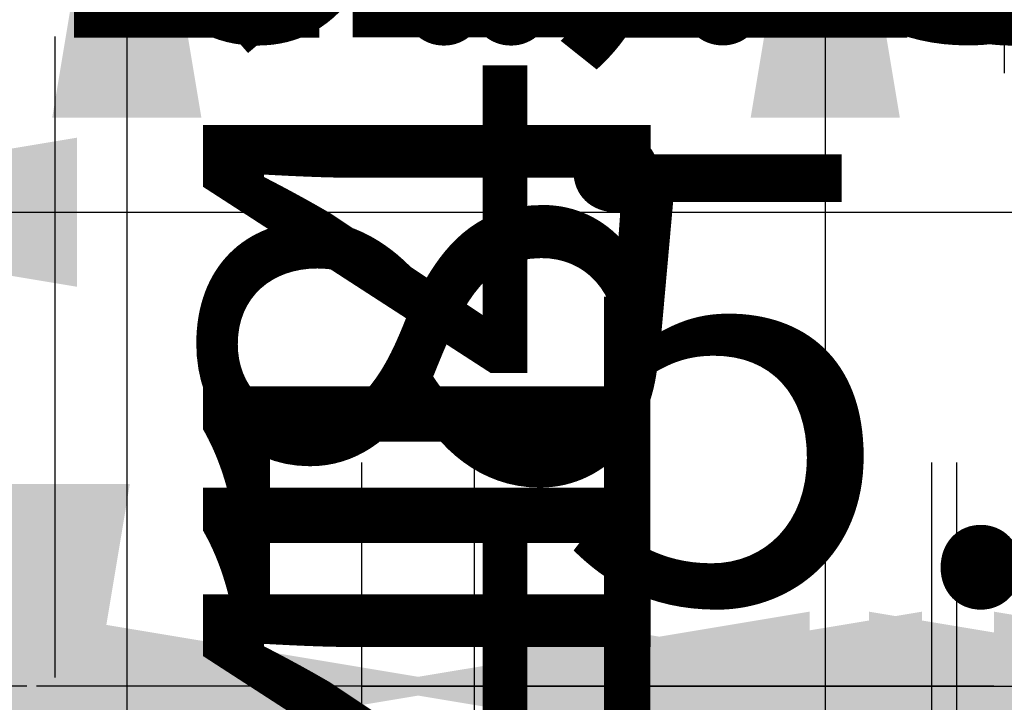
# Model space of a CAD drawing. Units: metres. Extents: x 782 to 1487, y 1262 to 7446.
# Tile 11 of 25: x 834.592 to 840.091, y 1284.539 to 1288.353. Entities that reach past the tile are written whole.
import ezdxf

# ---------------------------------------------------------------- set-up
doc = ezdxf.new("R2010")
doc.units = ezdxf.units.M
doc.layers.add('A-ANNO-DIMS', color=2, linetype='Continuous', lineweight=18)
doc.styles.get("Standard").update_dxf_attribs({"font": 'arial.ttf'})
doc.dimstyles.new('ISO-25', dxfattribs={"dimtxt": 2.5, "dimasz": 2.5, "dimexe": 1.25, "dimexo": 0.625, "dimtad": 1, "dimtxsty": 'Standard', "dimcen": 2.5, "dimadec": 0, "dimazin": 0, "dimtfac": 1, "dimtmove": 0, "dimatfit": 3, "dimfxl": 1, "dimarcsym": 0})

# ---------------------------------------------------------------- blocks, each defined once
blk = doc.blocks.new('*D88')
at = {"layer": 'A-ANNO-DIMS', "color": 0, "lineweight": -2, "transparency": 16777216}
for p, q in [((835.1905, 1307.3669), (835.1905, 1309.8669)), ((833.0382, 1304.8669), (836.4405, 1304.8669)), ((835.1905, 1304.8669), (835.1905, 1300.3378)), ((833.0381, 1300.3378), (836.4405, 1300.3378)), ((835.1905, 1297.8378), (835.1905, 1285.5459))]:
    blk.add_line(p, q, dxfattribs=at)
at = {"layer": 'A-ANNO-DIMS', "color": 0, "transparency": 16777216}
for points in [[(834.7738, 1307.3669), (835.6071, 1307.3669), (835.1905, 1304.8669)], [(834.7738, 1297.8378), (835.6071, 1297.8378), (835.1905, 1300.3378)]]:
    blk.add_solid(points, dxfattribs=at)
at = {"layer": 'Defpoints', "color": 0, "transparency": 16777216}
for p in [(832.4132, 1304.8669), (832.4131, 1300.3378), (835.1905, 1300.3378)]:
    blk.add_point(p, dxfattribs=at)
at = {"layer": 'A-ANNO-DIMS', "color": 0, "transparency": 16777216, "insert": (833.289, 1290.4419), "char_height": 2.5, "attachment_point": 5, "rotation": 90}
blk.add_mtext('4.529', dxfattribs=at)
blk = doc.blocks.new('*D89')
at = {"layer": 'A-ANNO-DIMS', "color": 0, "lineweight": -2, "transparency": 16777216}
for p, q in [((835.1905, 1302.8378), (835.1905, 1305.3378)), ((833.0381, 1300.3378), (836.4405, 1300.3378)), ((835.1905, 1300.3378), (835.1905, 1296.196)), ((833.0375, 1296.196), (836.4405, 1296.196)), ((835.1905, 1293.696), (835.1905, 1281.4347))]:
    blk.add_line(p, q, dxfattribs=at)
at = {"layer": 'A-ANNO-DIMS', "color": 0, "transparency": 16777216}
for points in [[(834.7738, 1302.8378), (835.6071, 1302.8378), (835.1905, 1300.3378)], [(834.7738, 1293.696), (835.6071, 1293.696), (835.1905, 1296.196)]]:
    blk.add_solid(points, dxfattribs=at)
at = {"layer": 'Defpoints', "color": 0, "transparency": 16777216}
for p in [(832.4131, 1300.3378), (832.4125, 1296.196), (835.1905, 1296.196)]:
    blk.add_point(p, dxfattribs=at)
at = {"layer": 'A-ANNO-DIMS', "color": 0, "transparency": 16777216, "insert": (833.3103, 1286.3153), "char_height": 2.5, "attachment_point": 5, "rotation": 90}
blk.add_mtext('4.142', dxfattribs=at)
blk = doc.blocks.new('*D90')
at = {"layer": 'A-ANNO-DIMS', "color": 0, "lineweight": -2, "transparency": 16777216}
for p, q in [((835.1905, 1298.696), (835.1905, 1301.196)), ((833.0375, 1296.196), (836.4405, 1296.196)), ((835.1905, 1296.196), (835.1905, 1293.6994)), ((833.0375, 1293.6994), (836.4405, 1293.6994)), ((835.1905, 1291.1994), (835.1905, 1280.9214))]:
    blk.add_line(p, q, dxfattribs=at)
at = {"layer": 'A-ANNO-DIMS', "color": 0, "transparency": 16777216}
for points in [[(834.7738, 1298.696), (835.6071, 1298.696), (835.1905, 1296.196)], [(834.7738, 1291.1994), (835.6071, 1291.1994), (835.1905, 1293.6994)]]:
    blk.add_solid(points, dxfattribs=at)
at = {"layer": 'Defpoints', "color": 0, "transparency": 16777216}
for p in [(832.4125, 1296.196), (832.4125, 1293.6994), (835.1905, 1293.6994)]:
    blk.add_point(p, dxfattribs=at)
at = {"layer": 'A-ANNO-DIMS', "color": 0, "transparency": 16777216, "insert": (833.289, 1284.8104), "char_height": 2.5, "attachment_point": 5, "rotation": 90}
blk.add_mtext('2.50', dxfattribs=at)
blk = doc.blocks.new('*D91')
at = {"layer": 'A-ANNO-DIMS', "color": 0, "lineweight": -2, "transparency": 16777216}
for p, q in [((835.1905, 1296.1994), (835.1905, 1298.6994)), ((833.0375, 1293.6994), (836.4405, 1293.6994)), ((835.1905, 1293.6994), (835.1905, 1293.0674)), ((833.0375, 1293.0674), (836.4405, 1293.0674)), ((835.1905, 1290.5674), (835.1905, 1278.4068))]:
    blk.add_line(p, q, dxfattribs=at)
at = {"layer": 'A-ANNO-DIMS', "color": 0, "transparency": 16777216}
for points in [[(834.7738, 1296.1994), (835.6071, 1296.1994), (835.1905, 1293.6994)], [(834.7738, 1290.5674), (835.6071, 1290.5674), (835.1905, 1293.0674)]]:
    blk.add_solid(points, dxfattribs=at)
at = {"layer": 'Defpoints', "color": 0, "transparency": 16777216}
for p in [(832.4125, 1293.6994), (832.4125, 1293.0674), (835.1905, 1293.0674)]:
    blk.add_point(p, dxfattribs=at)
at = {"layer": 'A-ANNO-DIMS', "color": 0, "transparency": 16777216, "insert": (833.2882, 1283.2371), "char_height": 2.5, "attachment_point": 5, "rotation": 90}
blk.add_mtext('0.632', dxfattribs=at)
blk = doc.blocks.new('*D92')
at = {"layer": 'A-ANNO-DIMS', "color": 0, "lineweight": -2, "transparency": 16777216}
for p, q in [((835.1905, 1295.5674), (835.1905, 1298.0674)), ((831.3406, 1293.0674), (836.4405, 1293.0674)), ((835.1905, 1293.0674), (835.1905, 1291.6863)), ((831.3406, 1291.6863), (836.4405, 1291.6863)), ((835.1905, 1289.1863), (835.1905, 1277.7181))]:
    blk.add_line(p, q, dxfattribs=at)
at = {"layer": 'A-ANNO-DIMS', "color": 0, "transparency": 16777216}
for points in [[(834.7738, 1295.5674), (835.6071, 1295.5674), (835.1905, 1293.0674)], [(834.7738, 1289.1863), (835.6071, 1289.1863), (835.1905, 1291.6863)]]:
    blk.add_solid(points, dxfattribs=at)
at = {"layer": 'Defpoints', "color": 0, "transparency": 16777216}
for p in [(830.7156, 1293.0674), (830.7156, 1291.6863), (835.1905, 1291.6863)]:
    blk.add_point(p, dxfattribs=at)
at = {"layer": 'A-ANNO-DIMS', "color": 0, "transparency": 16777216, "insert": (833.2882, 1282.2022), "char_height": 2.5, "attachment_point": 5, "rotation": 90}
blk.add_mtext('1.381', dxfattribs=at)
blk = doc.blocks.new('*D93')
at = {"layer": 'A-ANNO-DIMS', "color": 0, "lineweight": -2, "transparency": 16777216}
for p, q in [((835.1905, 1294.1863), (835.1905, 1296.6863)), ((831.3406, 1291.6863), (836.4405, 1291.6863)), ((835.1905, 1291.6863), (835.1905, 1290.3053)), ((831.3406, 1290.3053), (836.4405, 1290.3053)), ((835.1905, 1287.8053), (835.1905, 1276.337))]:
    blk.add_line(p, q, dxfattribs=at)
at = {"layer": 'A-ANNO-DIMS', "color": 0, "transparency": 16777216}
for points in [[(834.7738, 1294.1863), (835.6071, 1294.1863), (835.1905, 1291.6863)], [(834.7738, 1287.8053), (835.6071, 1287.8053), (835.1905, 1290.3053)]]:
    blk.add_solid(points, dxfattribs=at)
at = {"layer": 'Defpoints', "color": 0, "transparency": 16777216}
for p in [(830.7156, 1291.6863), (830.7156, 1290.3053), (835.1905, 1290.3053)]:
    blk.add_point(p, dxfattribs=at)
at = {"layer": 'A-ANNO-DIMS', "color": 0, "transparency": 16777216, "insert": (833.2882, 1280.8211), "char_height": 2.5, "attachment_point": 5, "rotation": 90}
blk.add_mtext('1.381', dxfattribs=at)
blk = doc.blocks.new('*D97')
at = {"layer": 'A-ANNO-DIMS', "color": 0, "lineweight": -2, "transparency": 16777216}
for p, q in [((827.9625, 1289.6803), (827.9625, 1286.0275)), ((829.1513, 1289.6803), (829.1513, 1286.0275)), ((825.4625, 1287.2775), (822.9625, 1287.2775)), ((827.9625, 1287.2775), (829.1513, 1287.2775)), ((831.6513, 1287.2775), (841.6649, 1287.2775))]:
    blk.add_line(p, q, dxfattribs=at)
at = {"layer": 'A-ANNO-DIMS', "color": 0, "transparency": 16777216}
for points in [[(825.4625, 1287.6941), (825.4625, 1286.8608), (827.9625, 1287.2775)], [(831.6513, 1287.6941), (831.6513, 1286.8608), (829.1513, 1287.2775)]]:
    blk.add_solid(points, dxfattribs=at)
at = {"layer": 'Defpoints', "color": 0, "transparency": 16777216}
for p in [(827.9625, 1290.3053), (829.1513, 1290.3053), (829.1513, 1287.2775)]:
    blk.add_point(p, dxfattribs=at)
at = {"layer": 'A-ANNO-DIMS', "color": 0, "transparency": 16777216, "insert": (837.9081, 1289.1789), "char_height": 2.5, "attachment_point": 5}
blk.add_mtext('1.19', dxfattribs=at)
blk = doc.blocks.new('*D98')
at = {"layer": 'A-ANNO-DIMS', "color": 0, "lineweight": -2, "transparency": 16777216}
for p, q in [((829.1513, 1289.6803), (829.1513, 1286.0275)), ((829.412, 1289.6803), (829.412, 1286.0275)), ((826.6513, 1287.2775), (824.1513, 1287.2775)), ((829.1513, 1287.2775), (829.412, 1287.2775)), ((831.912, 1287.2775), (842.1542, 1287.2775))]:
    blk.add_line(p, q, dxfattribs=at)
at = {"layer": 'A-ANNO-DIMS', "color": 0, "transparency": 16777216}
for points in [[(826.6513, 1287.6941), (826.6513, 1286.8608), (829.1513, 1287.2775)], [(831.912, 1287.6941), (831.912, 1286.8608), (829.412, 1287.2775)]]:
    blk.add_solid(points, dxfattribs=at)
at = {"layer": 'Defpoints', "color": 0, "transparency": 16777216}
for p in [(829.1513, 1290.3053), (829.412, 1290.3053), (829.412, 1287.2775)]:
    blk.add_point(p, dxfattribs=at)
at = {"layer": 'A-ANNO-DIMS', "color": 0, "transparency": 16777216, "insert": (838.2831, 1289.1789), "char_height": 2.5, "attachment_point": 5}
blk.add_mtext('0.26', dxfattribs=at)
blk = doc.blocks.new('*D99')
at = {"layer": 'A-ANNO-DIMS', "color": 0, "lineweight": -2, "transparency": 16777216}
for p, q in [((829.412, 1289.6803), (829.412, 1286.0275)), ((830.7156, 1289.6803), (830.7156, 1286.0275)), ((826.912, 1287.2775), (824.412, 1287.2775)), ((829.412, 1287.2775), (830.7156, 1287.2775)), ((833.2156, 1287.2775), (843.2156, 1287.2775))]:
    blk.add_line(p, q, dxfattribs=at)
at = {"layer": 'A-ANNO-DIMS', "color": 0, "transparency": 16777216}
for points in [[(826.912, 1287.6941), (826.912, 1286.8608), (829.412, 1287.2775)], [(833.2156, 1287.6941), (833.2156, 1286.8608), (830.7156, 1287.2775)]]:
    blk.add_solid(points, dxfattribs=at)
at = {"layer": 'Defpoints', "color": 0, "transparency": 16777216}
for p in [(829.412, 1290.3053), (830.7156, 1290.3053), (830.7156, 1287.2775)]:
    blk.add_point(p, dxfattribs=at)
at = {"layer": 'A-ANNO-DIMS', "color": 0, "transparency": 16777216, "insert": (839.4656, 1289.1798), "char_height": 2.5, "attachment_point": 5}
blk.add_mtext('1.30', dxfattribs=at)
blk = doc.blocks.new('*D100')
at = {"layer": 'A-ANNO-DIMS', "color": 0, "lineweight": -2, "transparency": 16777216}
for p, q in [((830.7156, 1289.6803), (830.7156, 1286.0275)), ((832.4125, 1289.6803), (832.4125, 1286.0275)), ((828.2156, 1287.2775), (825.7156, 1287.2775)), ((830.7156, 1287.2775), (832.4125, 1287.2775)), ((834.9125, 1287.2775), (846.8634, 1287.2775))]:
    blk.add_line(p, q, dxfattribs=at)
at = {"layer": 'A-ANNO-DIMS', "color": 0, "transparency": 16777216}
for points in [[(828.2156, 1287.6941), (828.2156, 1286.8608), (830.7156, 1287.2775)], [(834.9125, 1287.6941), (834.9125, 1286.8608), (832.4125, 1287.2775)]]:
    blk.add_solid(points, dxfattribs=at)
at = {"layer": 'Defpoints', "color": 0, "transparency": 16777216}
for p in [(830.7156, 1290.3053), (832.4125, 1290.3053), (832.4125, 1287.2775)]:
    blk.add_point(p, dxfattribs=at)
at = {"layer": 'A-ANNO-DIMS', "color": 0, "transparency": 16777216, "insert": (842.1379, 1289.1789), "char_height": 2.5, "attachment_point": 5}
blk.add_mtext('1.697', dxfattribs=at)
blk = doc.blocks.new('*D105')
at = {"layer": 'A-ANNO-DIMS', "color": 0, "lineweight": -2, "transparency": 16777216}
for p, q in [((840.0913, 1289.6803), (840.0913, 1288.0553)), ((841.2801, 1289.6803), (841.2801, 1288.0553)), ((837.5913, 1289.3053), (835.0913, 1289.3053)), ((840.0913, 1289.3053), (841.2801, 1289.3053)), ((843.7801, 1289.3053), (853.7938, 1289.3053))]:
    blk.add_line(p, q, dxfattribs=at)
at = {"layer": 'A-ANNO-DIMS', "color": 0, "transparency": 16777216}
for points in [[(837.5913, 1289.7219), (837.5913, 1288.8886), (840.0913, 1289.3053)], [(843.7801, 1289.7219), (843.7801, 1288.8886), (841.2801, 1289.3053)]]:
    blk.add_solid(points, dxfattribs=at)
at = {"layer": 'Defpoints', "color": 0, "transparency": 16777216}
for p in [(840.0913, 1290.3053), (841.2801, 1290.3053), (841.2801, 1289.3053)]:
    blk.add_point(p, dxfattribs=at)
at = {"layer": 'A-ANNO-DIMS', "color": 0, "transparency": 16777216, "insert": (850.037, 1291.2067), "char_height": 2.5, "attachment_point": 5}
blk.add_mtext('1.19', dxfattribs=at)
blk = doc.blocks.new('*D106')
at = {"layer": 'A-ANNO-DIMS', "color": 0, "lineweight": -2, "transparency": 16777216}
for p, q in [((841.2801, 1289.6803), (841.2801, 1288.0553)), ((841.5409, 1289.6803), (841.5409, 1288.0553)), ((838.7801, 1289.3053), (836.2801, 1289.3053)), ((841.2801, 1289.3053), (841.5409, 1289.3053)), ((844.0409, 1289.3053), (854.283, 1289.3053))]:
    blk.add_line(p, q, dxfattribs=at)
at = {"layer": 'A-ANNO-DIMS', "color": 0, "transparency": 16777216}
for points in [[(838.7801, 1289.7219), (838.7801, 1288.8886), (841.2801, 1289.3053)], [(844.0409, 1289.7219), (844.0409, 1288.8886), (841.5409, 1289.3053)]]:
    blk.add_solid(points, dxfattribs=at)
at = {"layer": 'Defpoints', "color": 0, "transparency": 16777216}
for p in [(841.2801, 1290.3053), (841.5409, 1290.3053), (841.5409, 1289.3053)]:
    blk.add_point(p, dxfattribs=at)
at = {"layer": 'A-ANNO-DIMS', "color": 0, "transparency": 16777216, "insert": (850.4119, 1291.2067), "char_height": 2.5, "attachment_point": 5}
blk.add_mtext('0.26', dxfattribs=at)
blk = doc.blocks.new('*D107')
at = {"layer": 'A-ANNO-DIMS', "color": 0, "lineweight": -2, "transparency": 16777216}
for p, q in [((841.5409, 1289.6803), (841.5409, 1288.0553)), ((842.8445, 1289.6803), (842.8445, 1288.0553)), ((839.0409, 1289.3053), (836.5409, 1289.3053)), ((841.5409, 1289.3053), (842.8445, 1289.3053)), ((845.3445, 1289.3053), (855.3445, 1289.3053))]:
    blk.add_line(p, q, dxfattribs=at)
at = {"layer": 'A-ANNO-DIMS', "color": 0, "transparency": 16777216}
for points in [[(839.0409, 1289.7219), (839.0409, 1288.8886), (841.5409, 1289.3053)], [(845.3445, 1289.7219), (845.3445, 1288.8886), (842.8445, 1289.3053)]]:
    blk.add_solid(points, dxfattribs=at)
at = {"layer": 'Defpoints', "color": 0, "transparency": 16777216}
for p in [(841.5409, 1290.3053), (842.8445, 1290.3053), (842.8445, 1289.3053)]:
    blk.add_point(p, dxfattribs=at)
at = {"layer": 'A-ANNO-DIMS', "color": 0, "transparency": 16777216, "insert": (851.5945, 1291.2076), "char_height": 2.5, "attachment_point": 5}
blk.add_mtext('1.30', dxfattribs=at)
blk = doc.blocks.new('*D108')
at = {"layer": 'A-ANNO-DIMS', "color": 0, "lineweight": -2, "transparency": 16777216}
for p, q in [((842.8445, 1289.6803), (842.8445, 1288.0553)), ((844.1849, 1289.6803), (844.1849, 1288.0553)), ((840.3445, 1289.3053), (837.8445, 1289.3053)), ((842.8445, 1289.3053), (844.1849, 1289.3053)), ((846.6849, 1289.3053), (856.6832, 1289.3053))]:
    blk.add_line(p, q, dxfattribs=at)
at = {"layer": 'A-ANNO-DIMS', "color": 0, "transparency": 16777216}
for points in [[(840.3445, 1289.7219), (840.3445, 1288.8886), (842.8445, 1289.3053)], [(846.6849, 1289.7219), (846.6849, 1288.8886), (844.1849, 1289.3053)]]:
    blk.add_solid(points, dxfattribs=at)
at = {"layer": 'Defpoints', "color": 0, "transparency": 16777216}
for p in [(842.8445, 1290.3053), (844.1849, 1290.3053), (844.1849, 1289.3053)]:
    blk.add_point(p, dxfattribs=at)
at = {"layer": 'A-ANNO-DIMS', "color": 0, "transparency": 16777216, "insert": (852.934, 1291.2076), "char_height": 2.5, "attachment_point": 5}
blk.add_mtext('1.34', dxfattribs=at)
blk = doc.blocks.new('*D110')
at = {"layer": 'A-ANNO-DIMS', "color": 0, "lineweight": -2, "transparency": 16777216}
for p, q in [((839.0913, 1307.6633), (839.0913, 1310.1633)), ((839.4663, 1305.1633), (837.8413, 1305.1633)), ((839.0913, 1305.1633), (839.0913, 1300.4593)), ((839.4663, 1300.4593), (837.8413, 1300.4593)), ((839.0913, 1297.9593), (839.0913, 1285.6827))]:
    blk.add_line(p, q, dxfattribs=at)
at = {"layer": 'A-ANNO-DIMS', "color": 0, "transparency": 16777216}
for points in [[(838.6746, 1307.6633), (839.508, 1307.6633), (839.0913, 1305.1633)], [(838.6746, 1297.9593), (839.508, 1297.9593), (839.0913, 1300.4593)]]:
    blk.add_solid(points, dxfattribs=at)
at = {"layer": 'Defpoints', "color": 0, "transparency": 16777216}
for p in [(840.0913, 1305.1633), (839.0913, 1300.4593), (840.0913, 1300.4593)]:
    blk.add_point(p, dxfattribs=at)
at = {"layer": 'A-ANNO-DIMS', "color": 0, "transparency": 16777216, "insert": (837.1899, 1290.571), "char_height": 2.5, "attachment_point": 5, "rotation": 90}
blk.add_mtext('4.704', dxfattribs=at)
blk = doc.blocks.new('*D111')
at = {"layer": 'A-ANNO-DIMS', "color": 0, "lineweight": -2, "transparency": 16777216}
for p, q in [((839.0913, 1302.9593), (839.0913, 1305.4593)), ((839.4663, 1300.4593), (837.8413, 1300.4593)), ((839.0913, 1300.4593), (839.0913, 1299.1153)), ((839.4663, 1299.1153), (837.8413, 1299.1153)), ((839.0913, 1296.6153), (839.0913, 1284.6747))]:
    blk.add_line(p, q, dxfattribs=at)
at = {"layer": 'A-ANNO-DIMS', "color": 0, "transparency": 16777216}
for points in [[(838.6746, 1302.9593), (839.508, 1302.9593), (839.0913, 1300.4593)], [(838.6746, 1296.6153), (839.508, 1296.6153), (839.0913, 1299.1153)]]:
    blk.add_solid(points, dxfattribs=at)
at = {"layer": 'Defpoints', "color": 0, "transparency": 16777216}
for p in [(840.0913, 1300.4593), (839.0913, 1299.1153), (840.0913, 1299.1153)]:
    blk.add_point(p, dxfattribs=at)
at = {"layer": 'A-ANNO-DIMS', "color": 0, "transparency": 16777216, "insert": (837.189, 1289.395), "char_height": 2.5, "attachment_point": 5, "rotation": 90}
blk.add_mtext('1.344', dxfattribs=at)
blk = doc.blocks.new('*D112')
at = {"layer": 'A-ANNO-DIMS', "color": 0, "lineweight": -2, "transparency": 16777216}
for p, q in [((839.0913, 1301.6153), (839.0913, 1304.1153)), ((839.4663, 1299.1153), (837.8413, 1299.1153)), ((839.0913, 1299.1153), (839.0913, 1293.0674)), ((839.4663, 1293.0674), (837.8413, 1293.0674)), ((839.0913, 1290.5674), (839.0913, 1278.3624))]:
    blk.add_line(p, q, dxfattribs=at)
at = {"layer": 'A-ANNO-DIMS', "color": 0, "transparency": 16777216}
for points in [[(838.6746, 1301.6153), (839.508, 1301.6153), (839.0913, 1299.1153)], [(838.6746, 1290.5674), (839.508, 1290.5674), (839.0913, 1293.0674)]]:
    blk.add_solid(points, dxfattribs=at)
at = {"layer": 'Defpoints', "color": 0, "transparency": 16777216}
for p in [(840.0913, 1299.1153), (839.0913, 1293.0674), (840.0913, 1293.0674)]:
    blk.add_point(p, dxfattribs=at)
at = {"layer": 'A-ANNO-DIMS', "color": 0, "transparency": 16777216, "insert": (837.1899, 1283.2149), "char_height": 2.5, "attachment_point": 5, "rotation": 90}
blk.add_mtext('6.048', dxfattribs=at)
blk = doc.blocks.new('*D113')
at = {"layer": 'A-ANNO-DIMS', "color": 0, "lineweight": -2, "transparency": 16777216}
for p, q in [((839.0913, 1295.5674), (839.0913, 1298.0674)), ((839.4663, 1293.0674), (837.8413, 1293.0674)), ((839.0913, 1293.0674), (839.0913, 1291.6863)), ((839.4663, 1291.6863), (837.8413, 1291.6863)), ((839.0913, 1289.1863), (839.0913, 1277.7181))]:
    blk.add_line(p, q, dxfattribs=at)
at = {"layer": 'A-ANNO-DIMS', "color": 0, "transparency": 16777216}
for points in [[(838.6746, 1295.5674), (839.508, 1295.5674), (839.0913, 1293.0674)], [(838.6746, 1289.1863), (839.508, 1289.1863), (839.0913, 1291.6863)]]:
    blk.add_solid(points, dxfattribs=at)
at = {"layer": 'Defpoints', "color": 0, "transparency": 16777216}
for p in [(840.0913, 1293.0674), (839.0913, 1291.6863), (840.0913, 1291.6863)]:
    blk.add_point(p, dxfattribs=at)
at = {"layer": 'A-ANNO-DIMS', "color": 0, "transparency": 16777216, "insert": (837.189, 1282.2022), "char_height": 2.5, "attachment_point": 5, "rotation": 90}
blk.add_mtext('1.381', dxfattribs=at)
blk = doc.blocks.new('*D114')
at = {"layer": 'A-ANNO-DIMS', "color": 0, "lineweight": -2, "transparency": 16777216}
for p, q in [((839.0913, 1294.1863), (839.0913, 1296.6863)), ((839.4663, 1291.6863), (837.8413, 1291.6863)), ((839.0913, 1291.6863), (839.0913, 1290.3053)), ((839.4663, 1290.3053), (837.8413, 1290.3053)), ((839.0913, 1287.8053), (839.0913, 1276.337))]:
    blk.add_line(p, q, dxfattribs=at)
at = {"layer": 'A-ANNO-DIMS', "color": 0, "transparency": 16777216}
for points in [[(838.6746, 1294.1863), (839.508, 1294.1863), (839.0913, 1291.6863)], [(838.6746, 1287.8053), (839.508, 1287.8053), (839.0913, 1290.3053)]]:
    blk.add_solid(points, dxfattribs=at)
at = {"layer": 'Defpoints', "color": 0, "transparency": 16777216}
for p in [(840.0913, 1291.6863), (839.0913, 1290.3053), (840.0913, 1290.3053)]:
    blk.add_point(p, dxfattribs=at)
at = {"layer": 'A-ANNO-DIMS', "color": 0, "transparency": 16777216, "insert": (837.189, 1280.8211), "char_height": 2.5, "attachment_point": 5, "rotation": 90}
blk.add_mtext('1.381', dxfattribs=at)
blk = doc.blocks.new('*D151')
at = {"layer": 'A-ANNO-DIMS', "color": 0, "lineweight": -2, "transparency": 16777216}
for p, q in [((839.686, 1273.6942), (839.686, 1285.8791)), ((841.835, 1273.6942), (841.835, 1285.8791)), ((837.186, 1284.6291), (834.686, 1284.6291)), ((839.686, 1284.6291), (841.835, 1284.6291)), ((844.335, 1284.6291), (856.569, 1284.6291))]:
    blk.add_line(p, q, dxfattribs=at)
at = {"layer": 'A-ANNO-DIMS', "color": 0, "transparency": 16777216}
for points in [[(837.186, 1285.0458), (837.186, 1284.2125), (839.686, 1284.6291)], [(844.335, 1285.0458), (844.335, 1284.2125), (841.835, 1284.6291)]]:
    blk.add_solid(points, dxfattribs=at)
at = {"layer": 'Defpoints', "color": 0, "transparency": 16777216}
for p in [(841.835, 1284.6291), (839.686, 1273.0692), (841.835, 1273.0692)]:
    blk.add_point(p, dxfattribs=at)
at = {"layer": 'A-ANNO-DIMS', "color": 0, "transparency": 16777216, "insert": (851.702, 1286.5306), "char_height": 2.5, "attachment_point": 5}
blk.add_mtext('2.149', dxfattribs=at)
blk = doc.blocks.new('*D152')
at = {"layer": 'A-ANNO-DIMS', "color": 0, "lineweight": -2, "transparency": 16777216}
for p, q in [((841.835, 1273.6942), (841.835, 1285.8791)), ((842.5333, 1273.6783), (842.5333, 1285.8791)), ((839.335, 1284.6291), (836.835, 1284.6291)), ((841.835, 1284.6291), (842.5333, 1284.6291)), ((845.0333, 1284.6291), (855.2686, 1284.6291))]:
    blk.add_line(p, q, dxfattribs=at)
at = {"layer": 'A-ANNO-DIMS', "color": 0, "transparency": 16777216}
for points in [[(839.335, 1285.0458), (839.335, 1284.2125), (841.835, 1284.6291)], [(845.0333, 1285.0458), (845.0333, 1284.2125), (842.5333, 1284.6291)]]:
    blk.add_solid(points, dxfattribs=at)
at = {"layer": 'Defpoints', "color": 0, "transparency": 16777216}
for p in [(842.5333, 1284.6291), (841.835, 1273.0692), (842.5333, 1273.0533)]:
    blk.add_point(p, dxfattribs=at)
at = {"layer": 'A-ANNO-DIMS', "color": 0, "transparency": 16777216, "insert": (851.4009, 1286.5306), "char_height": 2.5, "attachment_point": 5}
blk.add_mtext('0.70', dxfattribs=at)
blk = doc.blocks.new('*D153')
at = {"layer": 'A-ANNO-DIMS', "color": 0, "lineweight": -2, "transparency": 16777216}
for p, q in [((842.5333, 1273.6783), (842.5333, 1285.8791)), ((844.6687, 1273.6976), (844.6687, 1285.8791)), ((840.0333, 1284.6291), (837.5333, 1284.6291)), ((842.5333, 1284.6291), (844.6687, 1284.6291)), ((847.1687, 1284.6291), (857.445, 1284.6291))]:
    blk.add_line(p, q, dxfattribs=at)
at = {"layer": 'A-ANNO-DIMS', "color": 0, "transparency": 16777216}
for points in [[(840.0333, 1285.0458), (840.0333, 1284.2125), (842.5333, 1284.6291)], [(847.1687, 1285.0458), (847.1687, 1284.2125), (844.6687, 1284.6291)]]:
    blk.add_solid(points, dxfattribs=at)
at = {"layer": 'Defpoints', "color": 0, "transparency": 16777216}
for p in [(844.6687, 1284.6291), (842.5333, 1273.0533), (844.6687, 1273.0726)]:
    blk.add_point(p, dxfattribs=at)
at = {"layer": 'A-ANNO-DIMS', "color": 0, "transparency": 16777216, "insert": (853.5568, 1286.5093), "char_height": 2.5, "attachment_point": 5}
blk.add_mtext('2.14', dxfattribs=at)
blk = doc.blocks.new('*D154')
at = {"layer": 'A-ANNO-DIMS', "color": 0, "lineweight": -2, "transparency": 16777216}
for p, q in [((834.2886, 1275.5562), (834.2886, 1287.7305)), ((836.1342, 1273.0562), (833.0386, 1273.0562)), ((834.2886, 1269.1422), (834.2886, 1273.0562)), ((836.1187, 1269.1422), (833.0386, 1269.1422)), ((834.2886, 1266.6422), (834.2886, 1264.1422))]:
    blk.add_line(p, q, dxfattribs=at)
at = {"layer": 'A-ANNO-DIMS', "color": 0, "transparency": 16777216}
for points in [[(833.8719, 1275.5562), (834.7052, 1275.5562), (834.2886, 1273.0562)], [(833.8719, 1266.6422), (834.7052, 1266.6422), (834.2886, 1269.1422)]]:
    blk.add_solid(points, dxfattribs=at)
at = {"layer": 'Defpoints', "color": 0, "transparency": 16777216}
for p in [(834.2886, 1273.0562), (836.7592, 1273.0562), (836.7437, 1269.1422)]:
    blk.add_point(p, dxfattribs=at)
at = {"layer": 'A-ANNO-DIMS', "color": 0, "transparency": 16777216, "insert": (832.3863, 1282.8934), "char_height": 2.5, "attachment_point": 5, "rotation": 90}
blk.add_mtext('3.914', dxfattribs=at)
blk = doc.blocks.new('*D156')
at = {"layer": 'A-ANNO-DIMS', "color": 0, "lineweight": -2, "transparency": 16777216}
for p, q in [((836.5033, 1283.244), (836.5033, 1285.8791)), ((846.1759, 1283.244), (846.1759, 1285.8791)), ((839.0033, 1284.6291), (843.6759, 1284.6291)), ((846.1759, 1284.6291), (858.3621, 1284.6291))]:
    blk.add_line(p, q, dxfattribs=at)
at = {"layer": 'A-ANNO-DIMS', "color": 0, "transparency": 16777216}
for points in [[(839.0033, 1285.0458), (839.0033, 1284.2125), (836.5033, 1284.6291)], [(843.6759, 1285.0458), (843.6759, 1284.2125), (846.1759, 1284.6291)]]:
    blk.add_solid(points, dxfattribs=at)
at = {"layer": 'Defpoints', "color": 0, "transparency": 16777216}
for p in [(846.1759, 1284.6291), (836.5033, 1282.619), (846.1759, 1282.619)]:
    blk.add_point(p, dxfattribs=at)
at = {"layer": 'A-ANNO-DIMS', "color": 0, "transparency": 16777216, "insert": (853.519, 1286.5314), "char_height": 2.5, "attachment_point": 5}
blk.add_mtext('9.673', dxfattribs=at)
blk = doc.blocks.new('*D157')
at = {"layer": 'A-ANNO-DIMS', "color": 0, "lineweight": -2, "transparency": 16777216}
for p, q in [((834.2886, 1282.619), (834.2886, 1294.8189)), ((835.8783, 1282.619), (833.0386, 1282.619)), ((834.2886, 1278.7022), (834.2886, 1280.119)), ((835.8783, 1276.2022), (833.0386, 1276.2022))]:
    blk.add_line(p, q, dxfattribs=at)
at = {"layer": 'A-ANNO-DIMS', "color": 0, "transparency": 16777216}
for points in [[(833.8719, 1280.119), (834.7052, 1280.119), (834.2886, 1282.619)], [(833.8719, 1278.7022), (834.7052, 1278.7022), (834.2886, 1276.2022)]]:
    blk.add_solid(points, dxfattribs=at)
at = {"layer": 'Defpoints', "color": 0, "transparency": 16777216}
for p in [(834.2886, 1282.619), (836.5033, 1282.619), (836.5033, 1276.2022)]:
    blk.add_point(p, dxfattribs=at)
at = {"layer": 'A-ANNO-DIMS', "color": 0, "transparency": 16777216, "insert": (832.3871, 1289.9689), "char_height": 2.5, "attachment_point": 5, "rotation": 90}
blk.add_mtext('6.417', dxfattribs=at)
blk = doc.blocks.new('*D158')
at = {"layer": 'A-ANNO-DIMS', "color": 0, "lineweight": -2, "transparency": 16777216}
for p, q in [((836.5033, 1283.244), (836.5033, 1285.8791)), ((837.1321, 1282.6436), (837.1321, 1285.8791)), ((834.0033, 1284.6291), (831.5033, 1284.6291)), ((836.5033, 1284.6291), (837.1321, 1284.6291)), ((839.6321, 1284.6291), (849.876, 1284.6291))]:
    blk.add_line(p, q, dxfattribs=at)
at = {"layer": 'A-ANNO-DIMS', "color": 0, "transparency": 16777216}
for points in [[(834.0033, 1285.0458), (834.0033, 1284.2125), (836.5033, 1284.6291)], [(839.6321, 1285.0458), (839.6321, 1284.2125), (837.1321, 1284.6291)]]:
    blk.add_solid(points, dxfattribs=at)
at = {"layer": 'Defpoints', "color": 0, "transparency": 16777216}
for p in [(837.1321, 1284.6291), (836.5033, 1282.619), (837.1321, 1282.0186)]:
    blk.add_point(p, dxfattribs=at)
at = {"layer": 'A-ANNO-DIMS', "color": 0, "transparency": 16777216, "insert": (846.004, 1286.5314), "char_height": 2.5, "attachment_point": 5}
blk.add_mtext('0.63', dxfattribs=at)
blk = doc.blocks.new('*D159')
at = {"layer": 'A-ANNO-DIMS', "color": 0, "lineweight": -2, "transparency": 16777216}
for p, q in [((837.1321, 1282.6436), (837.1321, 1285.8791)), ((839.8262, 1282.6436), (839.8262, 1285.8791)), ((834.6321, 1284.6291), (832.1321, 1284.6291)), ((837.1321, 1284.6291), (839.8262, 1284.6291)), ((842.3262, 1284.6291), (854.5449, 1284.6291))]:
    blk.add_line(p, q, dxfattribs=at)
at = {"layer": 'A-ANNO-DIMS', "color": 0, "transparency": 16777216}
for points in [[(834.6321, 1285.0458), (834.6321, 1284.2125), (837.1321, 1284.6291)], [(842.3262, 1285.0458), (842.3262, 1284.2125), (839.8262, 1284.6291)]]:
    blk.add_solid(points, dxfattribs=at)
at = {"layer": 'Defpoints', "color": 0, "transparency": 16777216}
for p in [(839.8262, 1284.6291), (837.1321, 1282.0186), (839.8262, 1282.0186)]:
    blk.add_point(p, dxfattribs=at)
at = {"layer": 'A-ANNO-DIMS', "color": 0, "transparency": 16777216, "insert": (849.6855, 1286.5306), "char_height": 2.5, "attachment_point": 5}
blk.add_mtext('2.694', dxfattribs=at)
blk = doc.blocks.new('*D160')
at = {"layer": 'A-ANNO-DIMS', "color": 0, "lineweight": -2, "transparency": 16777216}
for p, q in [((839.8262, 1280.3128), (839.8262, 1285.8791)), ((841.2554, 1280.4442), (841.2554, 1285.8791)), ((837.3262, 1284.6291), (834.8262, 1284.6291)), ((839.8262, 1284.6291), (841.2554, 1284.6291)), ((843.7554, 1284.6291), (853.764, 1284.6291))]:
    blk.add_line(p, q, dxfattribs=at)
at = {"layer": 'A-ANNO-DIMS', "color": 0, "transparency": 16777216}
for points in [[(837.3262, 1285.0458), (837.3262, 1284.2125), (839.8262, 1284.6291)], [(843.7554, 1285.0458), (843.7554, 1284.2125), (841.2554, 1284.6291)]]:
    blk.add_solid(points, dxfattribs=at)
at = {"layer": 'Defpoints', "color": 0, "transparency": 16777216}
for p in [(841.2554, 1284.6291), (841.2554, 1279.8192), (839.8262, 1279.6878)]:
    blk.add_point(p, dxfattribs=at)
at = {"layer": 'A-ANNO-DIMS', "color": 0, "transparency": 16777216, "insert": (850.0097, 1286.5314), "char_height": 2.5, "attachment_point": 5}
blk.add_mtext('1.43', dxfattribs=at)
blk = doc.blocks.new('*D165')
at = {"layer": 'A-ANNO-DIMS', "color": 0, "lineweight": -2, "transparency": 16777216}
for p, q in [((826.3877, 1283.8847), (826.3877, 1285.3747)), ((832.0105, 1283.8847), (832.0105, 1285.3747)), ((823.8877, 1284.1247), (821.3877, 1284.1247)), ((826.3877, 1284.1247), (832.0105, 1284.1247)), ((834.5105, 1284.1247), (846.6967, 1284.1247))]:
    blk.add_line(p, q, dxfattribs=at)
at = {"layer": 'A-ANNO-DIMS', "color": 0, "transparency": 16777216}
for points in [[(823.8877, 1284.5413), (823.8877, 1283.708), (826.3877, 1284.1247)], [(834.5105, 1284.5413), (834.5105, 1283.708), (832.0105, 1284.1247)]]:
    blk.add_solid(points, dxfattribs=at)
at = {"layer": 'Defpoints', "color": 0, "transparency": 16777216}
for p in [(832.0105, 1284.1247), (826.3877, 1283.2597), (832.0105, 1283.2597)]:
    blk.add_point(p, dxfattribs=at)
at = {"layer": 'A-ANNO-DIMS', "color": 0, "transparency": 16777216, "insert": (841.8536, 1286.027), "char_height": 2.5, "attachment_point": 5}
blk.add_mtext('5.623', dxfattribs=at)
blk = doc.blocks.new('*D167')
at = {"layer": 'A-ANNO-DIMS', "color": 0, "lineweight": -2, "transparency": 16777216}
for p, q in [((834.7907, 1285.7597), (834.7907, 1288.2597)), ((832.6355, 1283.2597), (836.0407, 1283.2597)), ((834.7907, 1283.2597), (834.7907, 1282.1784)), ((831.7457, 1282.1784), (836.0407, 1282.1784)), ((834.7907, 1279.6784), (834.7907, 1269.6648))]:
    blk.add_line(p, q, dxfattribs=at)
at = {"layer": 'A-ANNO-DIMS', "color": 0, "transparency": 16777216}
for points in [[(834.3741, 1285.7597), (835.2074, 1285.7597), (834.7907, 1283.2597)], [(834.3741, 1279.6784), (835.2074, 1279.6784), (834.7907, 1282.1784)]]:
    blk.add_solid(points, dxfattribs=at)
at = {"layer": 'Defpoints', "color": 0, "transparency": 16777216}
for p in [(832.0105, 1283.2597), (831.1207, 1282.1784), (834.7907, 1282.1784)]:
    blk.add_point(p, dxfattribs=at)
at = {"layer": 'A-ANNO-DIMS', "color": 0, "transparency": 16777216, "insert": (832.8893, 1273.4216), "char_height": 2.5, "attachment_point": 5, "rotation": 90}
blk.add_mtext('1.08', dxfattribs=at)
blk = doc.blocks.new('*D168')
at = {"layer": 'A-ANNO-DIMS', "color": 0, "lineweight": -2, "transparency": 16777216}
for p, q in [((834.7907, 1284.6784), (834.7907, 1287.1784)), ((831.7457, 1282.1784), (836.0407, 1282.1784)), ((834.7907, 1282.1784), (834.7907, 1279.1214)), ((831.7457, 1279.1214), (836.0407, 1279.1214)), ((834.7907, 1276.6214), (834.7907, 1264.4369))]:
    blk.add_line(p, q, dxfattribs=at)
at = {"layer": 'A-ANNO-DIMS', "color": 0, "transparency": 16777216}
for points in [[(834.3741, 1284.6784), (835.2074, 1284.6784), (834.7907, 1282.1784)], [(834.3741, 1276.6214), (835.2074, 1276.6214), (834.7907, 1279.1214)]]:
    blk.add_solid(points, dxfattribs=at)
at = {"layer": 'Defpoints', "color": 0, "transparency": 16777216}
for p in [(831.1207, 1282.1784), (831.1207, 1279.1214), (834.7907, 1279.1214)]:
    blk.add_point(p, dxfattribs=at)
at = {"layer": 'A-ANNO-DIMS', "color": 0, "transparency": 16777216, "insert": (832.8885, 1269.2791), "char_height": 2.5, "attachment_point": 5, "rotation": 90}
blk.add_mtext('3.057', dxfattribs=at)

msp = doc.modelspace()

# ---------------------------------------------------------------- dimensions: what is measured, and where the dimension line sits
at = {"layer": 'A-ANNO-DIMS'}
for base, p1, p2, override, picture, middle in [((839.0913, 1300.4593), (840.0913, 1305.1633), (840.0913, 1300.4593), {"dimdec": 3, "dimlfac": 1, "dimrnd": 0, "dimzin": 0, "dimdsep": 46, "dimlunit": 2}, '*D110', (837.1899, 1290.571)), ((835.1905, 1300.3378), (832.4132, 1304.8669), (832.4131, 1300.3378), {"dimdec": 3, "dimlfac": 1, "dimrnd": 0, "dimzin": 0, "dimdsep": 46, "dimlunit": 2}, '*D88', (833.289, 1290.4419)), ((839.0913, 1299.1153), (840.0913, 1300.4593), (840.0913, 1299.1153), {"dimdec": 3, "dimlfac": 1, "dimrnd": 0, "dimzin": 0, "dimdsep": 46, "dimlunit": 2}, '*D111', (837.189, 1289.395)), ((835.1905, 1296.196), (832.4131, 1300.3378), (832.4125, 1296.196), {"dimdec": 3, "dimlfac": 1, "dimrnd": 0, "dimzin": 0, "dimdsep": 46, "dimlunit": 2}, '*D89', (833.3103, 1286.3153)), ((839.0913, 1293.0674), (840.0913, 1299.1153), (840.0913, 1293.0674), {"dimdec": 3, "dimlfac": 1, "dimrnd": 0, "dimzin": 0, "dimdsep": 46, "dimlunit": 2}, '*D112', (837.1899, 1283.2149)), ((835.1905, 1293.6994), (832.4125, 1296.196), (832.4125, 1293.6994), {"dimdec": 2, "dimlfac": 1, "dimrnd": 0, "dimzin": 0, "dimdsep": 46, "dimlunit": 2}, '*D90', (833.289, 1284.8104)), ((835.1905, 1293.0674), (832.4125, 1293.6994), (832.4125, 1293.0674), {"dimdec": 3, "dimlfac": 1, "dimrnd": 0, "dimzin": 0, "dimdsep": 46, "dimlunit": 2}, '*D91', (833.2882, 1283.2371)), ((835.1905, 1291.6863), (830.7156, 1293.0674), (830.7156, 1291.6863), {"dimdec": 3, "dimlfac": 1, "dimrnd": 0, "dimzin": 0, "dimdsep": 46, "dimlunit": 2}, '*D92', (833.2882, 1282.2022)), ((839.0913, 1291.6863), (840.0913, 1293.0674), (840.0913, 1291.6863), {"dimdec": 3, "dimlfac": 1, "dimrnd": 0, "dimzin": 0, "dimdsep": 46, "dimlunit": 2}, '*D113', (837.189, 1282.2022)), ((835.1905, 1290.3053), (830.7156, 1291.6863), (830.7156, 1290.3053), {"dimdec": 3, "dimlfac": 1, "dimrnd": 0, "dimzin": 0, "dimdsep": 46, "dimlunit": 2}, '*D93', (833.2882, 1280.8211)), ((839.0913, 1290.3053), (840.0913, 1291.6863), (840.0913, 1290.3053), {"dimdec": 3, "dimlfac": 1, "dimrnd": 0, "dimzin": 0, "dimdsep": 46, "dimlunit": 2}, '*D114', (837.189, 1280.8211)), ((834.2886, 1282.619), (836.5033, 1276.2022), (836.5033, 1282.619), {"dimdec": 3, "dimlfac": 1, "dimrnd": 0, "dimzin": 0, "dimdsep": 46, "dimlunit": 2}, '*D157', (832.3871, 1289.9689)), ((834.7907, 1282.1784), (832.0105, 1283.2597), (831.1207, 1282.1784), {"dimdec": 2, "dimlfac": 1, "dimrnd": 0, "dimzin": 0, "dimdsep": 46, "dimlunit": 2}, '*D167', (832.8893, 1273.4216)), ((834.2886, 1273.0562), (836.7437, 1269.1422), (836.7592, 1273.0562), {"dimdec": 3, "dimlfac": 1, "dimrnd": 0, "dimzin": 0, "dimdsep": 46, "dimlunit": 2}, '*D154', (832.3863, 1282.8934)), ((834.7907, 1279.1214), (831.1207, 1282.1784), (831.1207, 1279.1214), {"dimdec": 3, "dimlfac": 1, "dimrnd": 0, "dimzin": 0, "dimdsep": 46, "dimlunit": 2}, '*D168', (832.8885, 1269.2791))]:
    dim = msp.add_linear_dim(base=base, p1=p1, p2=p2, angle=90, dimstyle='ISO-25', override=override, dxfattribs=at)
    dim.commit()
    dim.dimension.update_dxf_attribs({"geometry": picture, "text_midpoint": middle})
for base, p1, p2, override, picture, middle in [((841.2801, 1289.3053), (840.0913, 1290.3053), (841.2801, 1290.3053), {"dimdec": 2, "dimlfac": 1, "dimrnd": 0, "dimzin": 0, "dimdsep": 46, "dimlunit": 2}, '*D105', (850.037, 1291.2067)), ((841.5409, 1289.3053), (841.2801, 1290.3053), (841.5409, 1290.3053), {"dimdec": 2, "dimlfac": 1, "dimrnd": 0, "dimzin": 0, "dimdsep": 46, "dimlunit": 2}, '*D106', (850.4119, 1291.2067)), ((842.8445, 1289.3053), (841.5409, 1290.3053), (842.8445, 1290.3053), {"dimdec": 2, "dimlfac": 1, "dimrnd": 0, "dimzin": 0, "dimdsep": 46, "dimlunit": 2}, '*D107', (851.5945, 1291.2076)), ((844.1849, 1289.3053), (842.8445, 1290.3053), (844.1849, 1290.3053), {"dimdec": 2, "dimlfac": 1, "dimrnd": 0, "dimzin": 0, "dimdsep": 46, "dimlunit": 2}, '*D108', (852.934, 1291.2076)), ((829.1513, 1287.2775), (827.9625, 1290.3053), (829.1513, 1290.3053), {"dimdec": 2, "dimlfac": 1, "dimrnd": 0, "dimzin": 0, "dimdsep": 46, "dimlunit": 2}, '*D97', (837.9081, 1289.1789)), ((829.412, 1287.2775), (829.1513, 1290.3053), (829.412, 1290.3053), {"dimdec": 2, "dimlfac": 1, "dimrnd": 0, "dimzin": 0, "dimdsep": 46, "dimlunit": 2}, '*D98', (838.2831, 1289.1789)), ((830.7156, 1287.2775), (829.412, 1290.3053), (830.7156, 1290.3053), {"dimdec": 2, "dimlfac": 1, "dimrnd": 0, "dimzin": 0, "dimdsep": 46, "dimlunit": 2}, '*D99', (839.4656, 1289.1798)), ((832.4125, 1287.2775), (830.7156, 1290.3053), (832.4125, 1290.3053), {"dimdec": 3, "dimlfac": 1, "dimrnd": 0, "dimzin": 0, "dimdsep": 46, "dimlunit": 2}, '*D100', (842.1379, 1289.1789)), ((837.1321, 1284.6291), (836.5033, 1282.619), (837.1321, 1282.0186), {"dimdec": 2, "dimlfac": 1, "dimrnd": 0, "dimzin": 0, "dimdsep": 46, "dimlunit": 2}, '*D158', (846.004, 1286.5314)), ((839.8262, 1284.6291), (837.1321, 1282.0186), (839.8262, 1282.0186), {"dimdec": 3, "dimlfac": 1, "dimrnd": 0, "dimzin": 0, "dimdsep": 46, "dimlunit": 2}, '*D159', (849.6855, 1286.5306)), ((841.835, 1284.6291), (839.686, 1273.0692), (841.835, 1273.0692), {"dimdec": 3, "dimlfac": 1, "dimrnd": 0, "dimzin": 0, "dimdsep": 46, "dimlunit": 2}, '*D151', (851.702, 1286.5306)), ((841.2554, 1284.6291), (839.8262, 1279.6878), (841.2554, 1279.8192), {"dimdec": 2, "dimlfac": 1, "dimrnd": 0, "dimzin": 0, "dimdsep": 46, "dimlunit": 2}, '*D160', (850.0097, 1286.5314)), ((846.1759, 1284.6291), (836.5033, 1282.619), (846.1759, 1282.619), {"dimdec": 3, "dimlfac": 1, "dimrnd": 0, "dimzin": 0, "dimdsep": 46, "dimlunit": 2}, '*D156', (853.519, 1286.5314)), ((842.5333, 1284.6291), (841.835, 1273.0692), (842.5333, 1273.0533), {"dimdec": 2, "dimlfac": 1, "dimrnd": 0, "dimzin": 0, "dimdsep": 46, "dimlunit": 2}, '*D152', (851.4009, 1286.5306)), ((844.6687, 1284.6291), (842.5333, 1273.0533), (844.6687, 1273.0726), {"dimdec": 2, "dimlfac": 1, "dimrnd": 0, "dimzin": 0, "dimdsep": 46, "dimlunit": 2}, '*D153', (853.5568, 1286.5093)), ((832.0105, 1284.1247), (826.3877, 1283.2597), (832.0105, 1283.2597), {"dimdec": 3, "dimlfac": 1, "dimrnd": 0, "dimzin": 0, "dimdsep": 46, "dimlunit": 2}, '*D165', (841.8536, 1286.027))]:
    dim = msp.add_linear_dim(base=base, p1=p1, p2=p2, dimstyle='ISO-25', override=override, dxfattribs=at)
    dim.commit()
    dim.dimension.update_dxf_attribs({"geometry": picture, "text_midpoint": middle})

doc.saveas('drawing.dxf')
